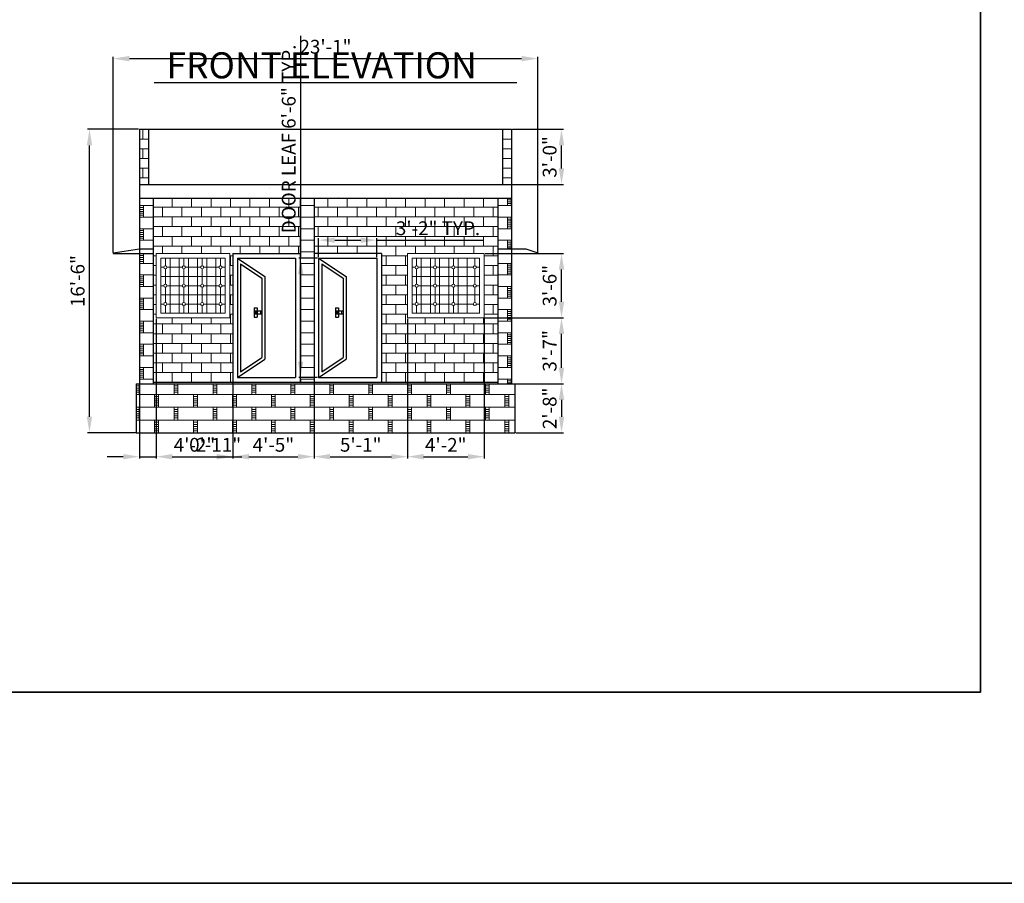
# Model space of a CAD drawing. Units: inches. Extents: x 1956 to 4770, y 1551 to 2596.
# Tile 8 of 10: x 2667 to 3310, y 1551 to 2115. Entities that reach past the tile are written whole.
import ezdxf

# ---------------------------------------------------------------- set-up
doc = ezdxf.new("R2010")
doc.units = ezdxf.units.IN
for name, color, linetype, lineweight in [('A-ANNO-DIMS', 2, 'Continuous', 18), ('A-ANNO-TITL', 6, 'Continuous', 25), ('A-ANNO-TTLB', 7, 'Continuous', 35), ('A-DOOR', 3, 'Continuous', 25), ('A-ELEV', 7, 'Continuous', 25), ('A-ELEV-PATT', 8, 'Continuous', 13), ('A-GLAZ', 4, 'Continuous', 18)]:
    doc.layers.add(name, color=color, linetype=linetype, lineweight=lineweight)
doc.styles.get("Standard").update_dxf_attribs({"font": 'arial.ttf'})
doc.dimstyles.new('ISO-25', dxfattribs={"dimtxt": 9, "dimasz": 10.5, "dimexe": 1.25, "dimexo": 0.625, "dimgap": 2, "dimtad": 1, "dimdec": 1, "dimlunit": 4, "dimtxsty": 'Standard', "dimcen": 2.5, "dimadec": 0, "dimazin": 0, "dimtfac": 1, "dimtdec": 1, "dimtmove": 0, "dimatfit": 3, "dimfxl": 1, "dimarcsym": 0})

# ---------------------------------------------------------------- blocks, each defined once
blk = doc.blocks.new('DOOR-ENTRY-PANEL-ELEV')
for p, q in [((0, 78), (38, 78)), ((0, 78), (0, 0)), ((0, 78), (18, 66)), ((38, 78), (38, 0)), ((2, 74.26), (16, 64.93)), ((2, 74.26), (2, 3.74)), ((16, 64.93), (16, 13.07)), ((18, 66), (18, 12)), ((11, 45.53), (11, 39.53)), ((11, 45.53), (13, 45.53)), ((13, 45.53), (13, 39.53)), ((11, 43.53), (16, 43.53)), ((11, 41.53), (16, 41.53)), ((11, 39.53), (13, 39.53)), ((12, 42.53), (11.64, 42.53)), ((12, 42.53), (12, 42.9)), ((12, 42.53), (12, 42.17)), ((12, 42.53), (12.36, 42.53)), ((15, 43.53), (15, 41.53)), ((16, 43.53), (16, 41.53)), ((2, 3.74), (16, 13.07)), ((0, 0), (18, 12)), ((0, 0), (38, 0))]:
    blk.add_line(p, q)
blk.add_circle((12, 42.53), 0.361)
blk = doc.blocks.new('*D41')
at = {"layer": 'A-ANNO-DIMS', "color": 0, "lineweight": -2, "transparency": 16777216}
for p, q in [((2850.27, 1959.25), (2850.27, 2104.31)), ((2861.35, 1959.25), (2849.02, 1959.25)), ((2850.27, 1891.75), (2850.27, 1948.75)), ((2861.35, 1881.25), (2849.02, 1881.25))]:
    blk.add_line(p, q, dxfattribs=at)
at = {"layer": 'A-ANNO-DIMS', "color": 0, "transparency": 16777216}
for points in [[(2848.52, 1948.75), (2852.02, 1948.75), (2850.27, 1959.25)], [(2848.52, 1891.75), (2852.02, 1891.75), (2850.27, 1881.25)]]:
    blk.add_solid(points, dxfattribs=at)
at = {"layer": 'Defpoints', "color": 0, "transparency": 16777216}
for p in [(2850.27, 1959.25), (2861.97, 1959.25), (2861.97, 1881.25)]:
    blk.add_point(p, dxfattribs=at)
at = {"layer": 'A-ANNO-DIMS', "color": 0, "transparency": 16777216, "insert": (2843.62, 2037.03), "char_height": 9, "attachment_point": 5, "rotation": 90}
blk.add_mtext('DOOR LEAF 6\'-6" TYP.', dxfattribs=at)
blk = doc.blocks.new('*D42')
at = {"layer": 'A-ANNO-DIMS', "color": 0, "lineweight": -2, "transparency": 16777216}
for p, q in [((2861.97, 1959.87), (2861.97, 1972.2)), ((2872.47, 1970.95), (2889.47, 1970.95)), ((2899.97, 1959.87), (2899.97, 1972.2)), ((2899.97, 1970.95), (2969.33, 1970.95))]:
    blk.add_line(p, q, dxfattribs=at)
at = {"layer": 'A-ANNO-DIMS', "color": 0, "transparency": 16777216}
for points in [[(2872.47, 1972.7), (2872.47, 1969.2), (2861.97, 1970.95)], [(2889.47, 1972.7), (2889.47, 1969.2), (2899.97, 1970.95)]]:
    blk.add_solid(points, dxfattribs=at)
at = {"layer": 'Defpoints', "color": 0, "transparency": 16777216}
for p in [(2899.97, 1970.95), (2861.97, 1959.25), (2899.97, 1959.25)]:
    blk.add_point(p, dxfattribs=at)
at = {"layer": 'A-ANNO-DIMS', "color": 0, "transparency": 16777216, "insert": (2939.9, 1977.55), "char_height": 9, "attachment_point": 5}
blk.add_mtext('3\'-2" TYP.', dxfattribs=at)
blk = doc.blocks.new('*D69')
at = {"layer": 'A-ANNO-DIMS', "color": 0, "lineweight": -2, "transparency": 16777216}
for p, q in [((2727.97, 1962.87), (2727.97, 2090.61)), ((2738.47, 2089.36), (2994.47, 2089.36)), ((3004.97, 1962.87), (3004.97, 2090.61))]:
    blk.add_line(p, q, dxfattribs=at)
at = {"layer": 'A-ANNO-DIMS', "color": 0, "transparency": 16777216}
for points in [[(2738.47, 2091.11), (2738.47, 2087.61), (2727.97, 2089.36)], [(2994.47, 2091.11), (2994.47, 2087.61), (3004.97, 2089.36)]]:
    blk.add_solid(points, dxfattribs=at)
at = {"layer": 'Defpoints', "color": 0, "transparency": 16777216}
for p in [(3004.97, 2089.36), (2727.97, 1962.25), (3004.97, 1962.25)]:
    blk.add_point(p, dxfattribs=at)
at = {"layer": 'A-ANNO-DIMS', "color": 0, "transparency": 16777216, "insert": (2866.47, 2095.95), "char_height": 9, "attachment_point": 5}
blk.add_mtext('23\'-1"', dxfattribs=at)
blk = doc.blocks.new('*D70')
at = {"layer": 'A-ANNO-DIMS', "color": 0, "lineweight": -2, "transparency": 16777216}
for p, q in [((2744.35, 2043.25), (2711.17, 2043.25)), ((2712.42, 1855.75), (2712.42, 2032.75)), ((2742.35, 1845.25), (2711.17, 1845.25))]:
    blk.add_line(p, q, dxfattribs=at)
at = {"layer": 'A-ANNO-DIMS', "color": 0, "transparency": 16777216}
for points in [[(2710.67, 2032.75), (2714.17, 2032.75), (2712.42, 2043.25)], [(2710.67, 1855.75), (2714.17, 1855.75), (2712.42, 1845.25)]]:
    blk.add_solid(points, dxfattribs=at)
at = {"layer": 'Defpoints', "color": 0, "transparency": 16777216}
for p in [(2712.42, 2043.25), (2744.97, 2043.25), (2742.97, 1845.25)]:
    blk.add_point(p, dxfattribs=at)
at = {"layer": 'A-ANNO-DIMS', "color": 0, "transparency": 16777216, "insert": (2705.83, 1944.25), "char_height": 9, "attachment_point": 5, "rotation": 90}
blk.add_mtext('16\'-6"', dxfattribs=at)
blk = doc.blocks.new('*D71')
at = {"layer": 'A-ANNO-DIMS', "color": 0, "lineweight": -2, "transparency": 16777216}
for p, q in [((2990.6, 1877.25), (3021.77, 1877.25)), ((3020.52, 1866.75), (3020.52, 1855.75)), ((2990.6, 1845.25), (3021.77, 1845.25))]:
    blk.add_line(p, q, dxfattribs=at)
at = {"layer": 'A-ANNO-DIMS', "color": 0, "transparency": 16777216}
for points in [[(3018.77, 1866.75), (3022.27, 1866.75), (3020.52, 1877.25)], [(3018.77, 1855.75), (3022.27, 1855.75), (3020.52, 1845.25)]]:
    blk.add_solid(points, dxfattribs=at)
at = {"layer": 'Defpoints', "color": 0, "transparency": 16777216}
for p in [(2989.97, 1877.25), (2989.97, 1845.25), (3020.52, 1845.25)]:
    blk.add_point(p, dxfattribs=at)
at = {"layer": 'A-ANNO-DIMS', "color": 0, "transparency": 16777216, "insert": (3013.93, 1861.25), "char_height": 9, "attachment_point": 5, "rotation": 90}
blk.add_mtext('2\'-8"', dxfattribs=at)
blk = doc.blocks.new('*D72')
at = {"layer": 'A-ANNO-DIMS', "color": 0, "lineweight": -2, "transparency": 16777216}
for p, q in [((2988.6, 2043.25), (3021.77, 2043.25)), ((3020.52, 2017.75), (3020.52, 2032.75)), ((2988.6, 2007.25), (3021.77, 2007.25))]:
    blk.add_line(p, q, dxfattribs=at)
at = {"layer": 'A-ANNO-DIMS', "color": 0, "transparency": 16777216}
for points in [[(3018.77, 2032.75), (3022.27, 2032.75), (3020.52, 2043.25)], [(3018.77, 2017.75), (3022.27, 2017.75), (3020.52, 2007.25)]]:
    blk.add_solid(points, dxfattribs=at)
at = {"layer": 'Defpoints', "color": 0, "transparency": 16777216}
for p in [(2987.97, 2043.25), (3020.52, 2043.25), (2987.97, 2007.25)]:
    blk.add_point(p, dxfattribs=at)
at = {"layer": 'A-ANNO-DIMS', "color": 0, "transparency": 16777216, "insert": (3013.93, 2025.25), "char_height": 9, "attachment_point": 5, "rotation": 90}
blk.add_mtext('3\'-0"', dxfattribs=at)
blk = doc.blocks.new('*D73')
at = {"layer": 'A-ANNO-DIMS', "color": 0, "lineweight": -2, "transparency": 16777216}
for p, q in [((2970.6, 1962.25), (3021.77, 1962.25)), ((3020.52, 1930.75), (3020.52, 1951.75)), ((2970.6, 1920.25), (3021.77, 1920.25))]:
    blk.add_line(p, q, dxfattribs=at)
at = {"layer": 'A-ANNO-DIMS', "color": 0, "transparency": 16777216}
for points in [[(3018.77, 1951.75), (3022.27, 1951.75), (3020.52, 1962.25)], [(3018.77, 1930.75), (3022.27, 1930.75), (3020.52, 1920.25)]]:
    blk.add_solid(points, dxfattribs=at)
at = {"layer": 'Defpoints', "color": 0, "transparency": 16777216}
for p in [(2969.97, 1962.25), (3020.52, 1962.25), (2969.97, 1920.25)]:
    blk.add_point(p, dxfattribs=at)
at = {"layer": 'A-ANNO-DIMS', "color": 0, "transparency": 16777216, "insert": (3013.93, 1941.25), "char_height": 9, "attachment_point": 5, "rotation": 90}
blk.add_mtext('3\'-6"', dxfattribs=at)
blk = doc.blocks.new('*D74')
at = {"layer": 'A-ANNO-DIMS', "color": 0, "lineweight": -2, "transparency": 16777216}
for p, q in [((2970.6, 1920.25), (3021.77, 1920.25)), ((3020.52, 1887.75), (3020.52, 1909.75)), ((2988.6, 1877.25), (3021.77, 1877.25))]:
    blk.add_line(p, q, dxfattribs=at)
at = {"layer": 'A-ANNO-DIMS', "color": 0, "transparency": 16777216}
for points in [[(3018.77, 1909.75), (3022.27, 1909.75), (3020.52, 1920.25)], [(3018.77, 1887.75), (3022.27, 1887.75), (3020.52, 1877.25)]]:
    blk.add_solid(points, dxfattribs=at)
at = {"layer": 'Defpoints', "color": 0, "transparency": 16777216}
for p in [(2969.97, 1920.25), (3020.52, 1920.25), (2987.97, 1877.25)]:
    blk.add_point(p, dxfattribs=at)
at = {"layer": 'A-ANNO-DIMS', "color": 0, "transparency": 16777216, "insert": (3013.93, 1898.75), "char_height": 9, "attachment_point": 5, "rotation": 90}
blk.add_mtext('3\'-7"', dxfattribs=at)
blk = doc.blocks.new('*D75')
at = {"layer": 'A-ANNO-DIMS', "color": 0, "lineweight": -2, "transparency": 16777216}
for p, q in [((2755.97, 1919.62), (2755.97, 1828.45)), ((2744.97, 1876.62), (2744.97, 1828.45)), ((2734.47, 1829.7), (2723.97, 1829.7)), ((2744.97, 1829.7), (2755.97, 1829.7)), ((2766.47, 1829.7), (2811.89, 1829.7))]:
    blk.add_line(p, q, dxfattribs=at)
at = {"layer": 'A-ANNO-DIMS', "color": 0, "transparency": 16777216}
for points in [[(2734.47, 1831.45), (2734.47, 1827.95), (2744.97, 1829.7)], [(2766.47, 1831.45), (2766.47, 1827.95), (2755.97, 1829.7)]]:
    blk.add_solid(points, dxfattribs=at)
at = {"layer": 'Defpoints', "color": 0, "transparency": 16777216}
for p in [(2755.97, 1920.25), (2744.97, 1877.25), (2755.97, 1829.7)]:
    blk.add_point(p, dxfattribs=at)
at = {"layer": 'A-ANNO-DIMS', "color": 0, "transparency": 16777216, "insert": (2794.43, 1836.29), "char_height": 9, "attachment_point": 5}
blk.add_mtext('0\'-11"', dxfattribs=at)
blk = doc.blocks.new('*D76')
at = {"layer": 'A-ANNO-DIMS', "color": 0, "lineweight": -2, "transparency": 16777216}
for p, q in [((2755.97, 1919.62), (2755.97, 1828.45)), ((2805.97, 1877.62), (2805.97, 1828.45)), ((2766.47, 1829.7), (2795.47, 1829.7))]:
    blk.add_line(p, q, dxfattribs=at)
at = {"layer": 'A-ANNO-DIMS', "color": 0, "transparency": 16777216}
for points in [[(2766.47, 1831.45), (2766.47, 1827.95), (2755.97, 1829.7)], [(2795.47, 1831.45), (2795.47, 1827.95), (2805.97, 1829.7)]]:
    blk.add_solid(points, dxfattribs=at)
at = {"layer": 'Defpoints', "color": 0, "transparency": 16777216}
for p in [(2755.97, 1920.25), (2805.97, 1878.25), (2805.97, 1829.7)]:
    blk.add_point(p, dxfattribs=at)
at = {"layer": 'A-ANNO-DIMS', "color": 0, "transparency": 16777216, "insert": (2780.97, 1836.22), "char_height": 9, "attachment_point": 5}
blk.add_mtext('4\'-2"', dxfattribs=at)
blk = doc.blocks.new('*D77')
at = {"layer": 'A-ANNO-DIMS', "color": 0, "lineweight": -2, "transparency": 16777216}
for p, q in [((2805.97, 1877.62), (2805.97, 1828.45)), ((2858.97, 1877.62), (2858.97, 1828.45)), ((2816.47, 1829.7), (2848.47, 1829.7))]:
    blk.add_line(p, q, dxfattribs=at)
at = {"layer": 'A-ANNO-DIMS', "color": 0, "transparency": 16777216}
for points in [[(2816.47, 1831.45), (2816.47, 1827.95), (2805.97, 1829.7)], [(2848.47, 1831.45), (2848.47, 1827.95), (2858.97, 1829.7)]]:
    blk.add_solid(points, dxfattribs=at)
at = {"layer": 'Defpoints', "color": 0, "transparency": 16777216}
for p in [(2805.97, 1878.25), (2858.97, 1878.25), (2858.97, 1829.7)]:
    blk.add_point(p, dxfattribs=at)
at = {"layer": 'A-ANNO-DIMS', "color": 0, "transparency": 16777216, "insert": (2832.47, 1836.28), "char_height": 9, "attachment_point": 5}
blk.add_mtext('4\'-5"', dxfattribs=at)
blk = doc.blocks.new('*D78')
at = {"layer": 'A-ANNO-DIMS', "color": 0, "lineweight": -2, "transparency": 16777216}
for p, q in [((2919.97, 1919.62), (2919.97, 1828.45)), ((2858.97, 1877.62), (2858.97, 1828.45)), ((2869.47, 1829.7), (2909.47, 1829.7))]:
    blk.add_line(p, q, dxfattribs=at)
at = {"layer": 'A-ANNO-DIMS', "color": 0, "transparency": 16777216}
for points in [[(2869.47, 1831.45), (2869.47, 1827.95), (2858.97, 1829.7)], [(2909.47, 1831.45), (2909.47, 1827.95), (2919.97, 1829.7)]]:
    blk.add_solid(points, dxfattribs=at)
at = {"layer": 'Defpoints', "color": 0, "transparency": 16777216}
for p in [(2919.97, 1920.25), (2858.97, 1878.25), (2919.97, 1829.7)]:
    blk.add_point(p, dxfattribs=at)
at = {"layer": 'A-ANNO-DIMS', "color": 0, "transparency": 16777216, "insert": (2889.47, 1836.29), "char_height": 9, "attachment_point": 5}
blk.add_mtext('5\'-1"', dxfattribs=at)
blk = doc.blocks.new('*D79')
at = {"layer": 'A-ANNO-DIMS', "color": 0, "lineweight": -2, "transparency": 16777216}
for p, q in [((2919.97, 1919.62), (2919.97, 1828.45)), ((2969.97, 1919.62), (2969.97, 1828.45)), ((2930.47, 1829.7), (2959.47, 1829.7))]:
    blk.add_line(p, q, dxfattribs=at)
at = {"layer": 'A-ANNO-DIMS', "color": 0, "transparency": 16777216}
for points in [[(2930.47, 1831.45), (2930.47, 1827.95), (2919.97, 1829.7)], [(2959.47, 1831.45), (2959.47, 1827.95), (2969.97, 1829.7)]]:
    blk.add_solid(points, dxfattribs=at)
at = {"layer": 'Defpoints', "color": 0, "transparency": 16777216}
for p in [(2919.97, 1920.25), (2969.97, 1920.25), (2969.97, 1829.7)]:
    blk.add_point(p, dxfattribs=at)
at = {"layer": 'A-ANNO-DIMS', "color": 0, "transparency": 16777216, "insert": (2944.97, 1836.22), "char_height": 9, "attachment_point": 5}
blk.add_mtext('4\'-2"', dxfattribs=at)

msp = doc.modelspace()

# ---------------------------------------------------------------- hatches: boundary and pattern name
at = {"layer": 'A-ELEV-PATT'}
h = msp.add_hatch(dxfattribs=at)
h.set_pattern_fill('BRICK', color=256)
h.set_pattern_definition([(0, (486.7216, 462.123), (0, 6.35), []), (90, (486.722, 462.123), (-12.7, 8e-16), [6.35, -6.35]), (90, (493.072, 462.123), (-12.7, 8e-16), [-6.35, 6.35])])
h.paths.add_polyline_path([(2805.97, 1962.25), (2849.97, 1962.25), (2849.97, 1998.25), (2753.97, 1998.25), (2753.97, 1878.25), (2805.97, 1878.25)])
h.paths.add_polyline_path([(2803.97, 1962.25), (2803.97, 1920.25), (2755.97, 1920.25), (2755.97, 1962.25)], flags=16)
h.paths.add_polyline_path([(2800.97, 1959.25), (2800.97, 1923.25), (2758.97, 1923.25), (2758.97, 1959.25)], flags=0)
h.paths.add_polyline_path([(2799, 1953.25, -0.414214), (2797.97, 1952.23), (2797.97, 1942.27, -0.414214), (2799, 1941.25, -0.414214), (2797.97, 1940.23), (2797.97, 1930.27, -0.414214), (2799, 1929.25, -1), (2796.95, 1929.25), (2787, 1929.25, -1), (2784.95, 1929.25), (2775, 1929.25, -1), (2772.95, 1929.25), (2763, 1929.25, -1), (2760.95, 1929.25, -0.414214), (2761.97, 1930.27), (2761.97, 1940.23, -0.414214), (2760.95, 1941.25, -0.414214), (2761.97, 1942.27), (2761.97, 1952.23, -0.414214), (2760.95, 1953.25, -1), (2763, 1953.25), (2772.95, 1953.25, -1), (2775, 1953.25), (2784.95, 1953.25, -1), (2787, 1953.25), (2796.95, 1953.25, -1)], flags=0)
h.paths.add_polyline_path([(2794.97, 1935.25), (2764.97, 1935.25), (2764.97, 1947.25), (2794.97, 1947.25)], flags=0)
h.paths.add_polyline_path([(2787, 1941.25, -1), (2784.95, 1941.25), (2775, 1941.25, -1), (2772.95, 1941.25, -1), (2775, 1941.25), (2784.95, 1941.25, -1)], flags=0)
h.paths.add_polyline_path([(2902.97, 1962.25), (2902.97, 1878.25), (2978.97, 1878.25), (2978.97, 1998.25), (2858.97, 1998.25), (2858.97, 1962.25)])
h.paths.add_polyline_path([(2919.97, 1962.25), (2969.97, 1962.25), (2969.97, 1920.25), (2919.97, 1920.25)], flags=16)
h.paths.add_polyline_path([(2922.97, 1959.25), (2966.97, 1959.25), (2966.97, 1923.25), (2922.97, 1923.25)], flags=0)
h.paths.add_polyline_path([(2927, 1953.25), (2936.95, 1953.25, -1), (2939, 1953.25), (2948.95, 1953.25, -1), (2951, 1953.25), (2962.95, 1953.25, -1), (2965, 1953.25, -0.414214), (2963.97, 1952.23), (2963.97, 1942.27, -0.414214), (2965, 1941.25, -0.414214), (2963.97, 1940.23), (2963.97, 1930.27, -0.414214), (2965, 1929.25, -1), (2962.95, 1929.25), (2951, 1929.25, -1), (2948.95, 1929.25), (2939, 1929.25, -1), (2936.95, 1929.25), (2927, 1929.25, -1), (2924.95, 1929.25, -0.414214), (2925.97, 1930.27), (2925.97, 1940.23, -0.414214), (2924.95, 1941.25, -0.414214), (2925.97, 1942.27), (2925.97, 1952.23, -0.414214), (2924.95, 1953.25, -1)], flags=0)
h.paths.add_polyline_path([(2928.97, 1947.25), (2958.97, 1947.25), (2958.97, 1935.25), (2928.97, 1935.25)], flags=0)
h.paths.add_polyline_path([(2939, 1941.25), (2948.95, 1941.25, -1), (2951, 1941.25, -1), (2948.95, 1941.25), (2939, 1941.25, -1), (2936.95, 1941.25, -1)], flags=0)
h.paths.add_polyline_path([(2750.97, 2043.25), (2744.97, 2043.25), (2744.97, 2007.25), (2750.97, 2007.25)])
h.paths.add_polyline_path([(2987.97, 2043.25), (2981.97, 2043.25), (2981.97, 2007.25), (2987.97, 2007.25)])
h = msp.add_hatch(dxfattribs=at)
h.set_pattern_fill('AR-CONC', color=256, scale=0.9)
h.set_pattern_definition([(50, (486.72, 462.12), (163.966, -14.345), [17.145, -188.595]), (355, (486.72, 462.12), (-31.719, 171.951), [13.716, -150.8765]), (100.4514, (500.39, 460.93), (132.247, 157.606), [14.571, -160.281]), (46.184, (486.72, 507.84), (243.971, -37.838), [25.718, -282.892]), (96.636, (507.05, 504.7), (213.664, 222.684), [21.857, -240.422]), (351.184, (486.72, 507.84), (213.664, 222.684), [20.574, -226.314]), (21, (509.58, 496.41), (136.453, -92.0387), [17.145, -188.595]), (326, (509.58, 496.41), (55.622, 165.769), [13.716, -150.876]), (71.4514, (520.95, 488.74), (192.075, 73.7305), [14.571, -160.281]), (37.5, (486.72, 462.123), (2.7797, 76.0995), [0, -149.0472, 0, -153.162, 0, -151.4475]), (7.5, (486.72, 462.12), (60.1377, 90.1625), [0, -87.3252, 0, -145.6182, 0, -57.7215]), (327.5, (435.744, 462.123), (122.0315, -5.1559), [0, -57.15, 0, -178.308, 0, -236.601]), (317.5, (412.88, 462.12), (133.3163, 22.884), [0, -74.295, 0, -118.4148, 0, -168.021])])
h.paths.add_polyline_path([(2849.97, 1998.25), (2987.97, 1998.25), (2987.97, 2007.25), (2744.97, 2007.25), (2744.97, 1998.25)])
h = msp.add_hatch(dxfattribs=at)
h.set_pattern_fill('BRSTONE', color=256, scale=0.9)
h.set_pattern_definition([(0, (486.7216, 462.123), (0, 7.5438), []), (90, (507.296, 462.123), (-11.43, 7.5438), [7.5438, -7.5438]), (90, (505.01, 462.123), (-11.43, 7.5438), [7.5438, -7.5438]), (0, (507.2956, 463.3805), (11.43, 7.5438), [-20.574, 2.286]), (0, (507.2956, 464.638), (11.43, 7.5438), [-20.574, 2.286]), (0, (507.2956, 465.895), (11.43, 7.5438), [-20.574, 2.286]), (0, (507.2956, 467.1524), (11.43, 7.5438), [-20.574, 2.286]), (0, (507.2956, 468.41), (11.43, 7.5438), [-20.574, 2.286])])
h.paths.add_polyline_path([(2744.97, 1877.25), (2753.97, 1877.25), (2753.97, 1962.25), (2744.97, 1962.25)])
h.paths.add_polyline_path([(2744.97, 1965.25), (2753.97, 1965.25), (2753.97, 1998.25), (2744.97, 1998.25)])
h.paths.add_polyline_path([(2849.97, 1998.25), (2849.97, 1878.25), (2858.97, 1878.25), (2858.97, 1998.25)])
h.paths.add_polyline_path([(2987.97, 1998.25), (2978.97, 1998.25), (2978.97, 1965.25), (2987.97, 1965.25)])
h.paths.add_polyline_path([(2978.97, 1877.25), (2987.97, 1877.25), (2987.97, 1962.25), (2978.97, 1962.25)])
h = msp.add_hatch(dxfattribs=at)
h.set_pattern_fill('BRSTONE', color=256)
h.set_pattern_definition([(0, (486.7216, 462.123), (0, 8.382), []), (90, (509.582, 462.123), (-12.7, 8.382), [8.382, -8.382]), (90, (507.042, 462.123), (-12.7, 8.382), [8.382, -8.382]), (0, (509.5816, 463.52), (12.7, 8.382), [-22.86, 2.54]), (0, (509.5816, 464.917), (12.7, 8.382), [-22.86, 2.54]), (0, (509.5816, 466.314), (12.7, 8.382), [-22.86, 2.54]), (0, (509.5816, 467.711), (12.7, 8.382), [-22.86, 2.54]), (0, (509.5816, 469.108), (12.7, 8.382), [-22.86, 2.54])])
h.paths.add_polyline_path([(2989.97, 1877.25), (2742.97, 1877.25), (2742.97, 1845.25), (2989.97, 1845.25)])

# ---------------------------------------------------------------- linework, layer by layer
at = {"layer": 'A-ANNO-TITL'}
msp.add_line((2754.74, 2073.81), (2991.37, 2073.81), dxfattribs=at)
at = {"layer": 'A-ANNO-TTLB'}
for points in [[(1955.79, 2596.29), (4769.89, 2596.29), (4769.89, 1551.4), (1955.79, 1551.4)], [(2042.64, 2439.33), (3293.93, 2439.33), (3293.93, 1676.04), (2042.64, 1676.04)]]:
    msp.add_lwpolyline(points, close=True, dxfattribs=at)
at = {"layer": 'A-DOOR'}
for p, q in [((2805.97, 1962.25), (2805.97, 1878.25)), ((2805.97, 1962.25), (2849.97, 1962.25)), ((2805.97, 1962.25), (2805.97, 1878.25)), ((2902.97, 1962.25), (2858.97, 1962.25)), ((2902.97, 1962.25), (2902.97, 1878.25))]:
    msp.add_line(p, q, dxfattribs=at)
at = {"layer": 'A-ELEV'}
for p, q in [((2744.97, 2043.25), (2744.97, 1877.25)), ((2744.97, 2043.25), (2987.97, 2043.25)), ((2750.97, 2043.25), (2750.97, 2007.25)), ((2981.97, 2043.25), (2981.97, 2007.25)), ((2987.97, 2043.25), (2987.97, 1877.25)), ((2744.97, 2007.25), (2987.97, 2007.25)), ((2744.97, 1998.25), (2849.97, 1998.25)), ((2753.97, 1998.25), (2753.97, 1877.25)), ((2849.97, 1998.25), (2849.97, 1878.25)), ((2849.97, 1998.25), (2987.97, 1998.25)), ((2858.97, 1998.25), (2858.97, 1878.25)), ((2978.97, 1998.25), (2978.97, 1877.25)), ((2727.97, 1962.75), (2744.97, 1965.25)), ((2727.97, 1962.75), (2727.97, 1962.25)), ((2727.97, 1962.25), (2753.97, 1962.25)), ((2744.97, 1965.25), (2753.97, 1965.25)), ((2978.97, 1965.25), (2997.25, 1965.25)), ((2978.97, 1962.25), (3004.97, 1962.25)), ((2997.25, 1965.25), (3004.97, 1962.75)), ((3004.97, 1962.75), (3004.97, 1962.25)), ((2969.97, 1920.25), (2987.97, 1920.25)), ((2742.97, 1877.25), (2989.97, 1877.25)), ((2742.97, 1877.25), (2742.97, 1845.25)), ((2753.97, 1878.25), (2978.97, 1878.25)), ((2987.97, 1877.25), (2989.97, 1877.25)), ((2989.97, 1877.25), (2989.97, 1845.25)), ((2742.97, 1845.25), (2989.97, 1845.25))]:
    msp.add_line(p, q, dxfattribs=at)
at = {"layer": 'A-GLAZ'}
for p, q in [((2755.97, 1962.25), (2803.97, 1962.25)), ((2755.97, 1962.25), (2755.97, 1920.25)), ((2803.97, 1962.25), (2803.97, 1920.25)), ((2919.97, 1962.25), (2969.97, 1962.25)), ((2919.97, 1962.25), (2919.97, 1920.25)), ((2969.97, 1962.25), (2969.97, 1920.25)), ((2758.97, 1959.25), (2800.97, 1959.25)), ((2758.97, 1959.25), (2758.97, 1923.25)), ((2761.97, 1959.25), (2761.97, 1954.27)), ((2764.97, 1959.25), (2764.97, 1923.25)), ((2770.97, 1959.25), (2770.97, 1923.25)), ((2773.97, 1959.25), (2773.97, 1954.27)), ((2776.97, 1959.25), (2776.97, 1923.25)), ((2782.97, 1959.25), (2782.97, 1923.25)), ((2785.97, 1959.25), (2785.97, 1954.27)), ((2788.97, 1959.25), (2788.97, 1923.25)), ((2794.97, 1959.25), (2794.97, 1923.25)), ((2797.97, 1959.25), (2797.97, 1954.27)), ((2800.97, 1959.25), (2800.97, 1923.25)), ((2922.97, 1959.25), (2966.97, 1959.25)), ((2922.97, 1959.25), (2922.97, 1923.25)), ((2925.97, 1959.25), (2925.97, 1954.27)), ((2928.97, 1959.25), (2928.97, 1923.25)), ((2934.97, 1959.25), (2934.97, 1923.25)), ((2937.97, 1959.25), (2937.97, 1954.27)), ((2940.97, 1959.25), (2940.97, 1923.25)), ((2946.97, 1959.25), (2946.97, 1923.25)), ((2949.97, 1959.25), (2949.97, 1954.27)), ((2952.97, 1959.25), (2952.97, 1923.25)), ((2958.97, 1959.25), (2958.97, 1923.25)), ((2963.97, 1959.25), (2963.97, 1954.27)), ((2966.97, 1959.25), (2966.97, 1923.25)), ((2758.97, 1953.25), (2760.95, 1953.25)), ((2761.97, 1952.23), (2761.97, 1942.27)), ((2763, 1953.25), (2772.95, 1953.25)), ((2773.97, 1952.23), (2773.97, 1942.27)), ((2775, 1953.25), (2784.95, 1953.25)), ((2785.97, 1952.23), (2785.97, 1942.27)), ((2787, 1953.25), (2796.95, 1953.25)), ((2797.97, 1952.23), (2797.97, 1942.27)), ((2799, 1953.25), (2800.97, 1953.25)), ((2922.97, 1953.25), (2924.95, 1953.25)), ((2925.97, 1952.23), (2925.97, 1942.27)), ((2927, 1953.25), (2936.95, 1953.25)), ((2937.97, 1952.23), (2937.97, 1942.27)), ((2939, 1953.25), (2948.95, 1953.25)), ((2949.97, 1952.23), (2949.97, 1942.27)), ((2951, 1953.25), (2962.95, 1953.25)), ((2963.97, 1952.23), (2963.97, 1942.27)), ((2965, 1953.25), (2966.97, 1953.25)), ((2758.97, 1947.25), (2800.97, 1947.25)), ((2758.97, 1941.25), (2760.95, 1941.25)), ((2763, 1941.25), (2772.95, 1941.25)), ((2775, 1941.25), (2784.95, 1941.25)), ((2787, 1941.25), (2796.95, 1941.25)), ((2799, 1941.25), (2800.97, 1941.25)), ((2922.97, 1947.25), (2966.97, 1947.25)), ((2922.97, 1941.25), (2924.95, 1941.25)), ((2927, 1941.25), (2936.95, 1941.25)), ((2939, 1941.25), (2948.95, 1941.25)), ((2951, 1941.25), (2962.95, 1941.25)), ((2965, 1941.25), (2966.97, 1941.25)), ((2758.97, 1935.25), (2800.97, 1935.25)), ((2761.97, 1940.23), (2761.97, 1930.27)), ((2773.97, 1940.23), (2773.97, 1930.27)), ((2785.97, 1940.23), (2785.97, 1930.27)), ((2797.97, 1940.23), (2797.97, 1930.27)), ((2922.97, 1935.25), (2966.97, 1935.25)), ((2925.97, 1940.23), (2925.97, 1930.27)), ((2937.97, 1940.23), (2937.97, 1930.27)), ((2949.97, 1940.23), (2949.97, 1930.27)), ((2963.97, 1940.23), (2963.97, 1930.27)), ((2758.97, 1929.25), (2760.95, 1929.25)), ((2761.97, 1928.23), (2761.97, 1923.25)), ((2763, 1929.25), (2772.95, 1929.25)), ((2773.97, 1928.23), (2773.97, 1923.25)), ((2775, 1929.25), (2784.95, 1929.25)), ((2785.97, 1928.23), (2785.97, 1923.25)), ((2787, 1929.25), (2796.95, 1929.25)), ((2797.97, 1928.23), (2797.97, 1923.25)), ((2799, 1929.25), (2800.97, 1929.25)), ((2922.97, 1929.25), (2924.95, 1929.25)), ((2925.97, 1928.23), (2925.97, 1923.25)), ((2927, 1929.25), (2936.95, 1929.25)), ((2937.97, 1928.23), (2937.97, 1923.25)), ((2939, 1929.25), (2948.95, 1929.25)), ((2949.97, 1928.23), (2949.97, 1923.25)), ((2951, 1929.25), (2962.95, 1929.25)), ((2965, 1929.25), (2966.97, 1929.25)), ((2758.97, 1923.25), (2800.97, 1923.25)), ((2922.97, 1923.25), (2966.97, 1923.25)), ((2755.97, 1920.25), (2803.97, 1920.25)), ((2919.97, 1920.25), (2969.97, 1920.25))]:
    msp.add_line(p, q, dxfattribs=at)
for centre in [(2761.97, 1953.25), (2773.97, 1953.25), (2785.97, 1953.25), (2797.97, 1953.25), (2925.97, 1953.25), (2937.97, 1953.25), (2949.97, 1953.25), (2963.97, 1953.25), (2761.97, 1941.25), (2773.97, 1941.25), (2785.97, 1941.25), (2797.97, 1941.25), (2925.97, 1941.25), (2937.97, 1941.25), (2949.97, 1941.25), (2963.97, 1941.25), (2761.97, 1929.25), (2773.97, 1929.25), (2785.97, 1929.25), (2797.97, 1929.25), (2925.97, 1929.25), (2937.97, 1929.25), (2949.97, 1929.25), (2963.97, 1929.25)]:
    msp.add_circle(centre, 1.02, dxfattribs=at)

# ---------------------------------------------------------------- block references
at = {"layer": 'A-DOOR'}
for p in [(2808.97, 1881.25), (2861.97, 1881.25)]:
    msp.add_blockref('DOOR-ENTRY-PANEL-ELEV', p, dxfattribs=at)

# ---------------------------------------------------------------- texts
at = {"layer": 'A-ANNO-TITL'}
msp.add_text(' FRONT ELEVATION ', height=17, dxfattribs=at).set_placement((2757.42, 2076.5))

# ---------------------------------------------------------------- dimensions: what is measured, and where the dimension line sits
at = {"layer": 'A-ANNO-DIMS'}
for base, p1, p2, picture, middle in [((3004.97, 2089.36), (2727.97, 1962.25), (3004.97, 1962.25), '*D69', (2866.47, 2095.95)), ((2755.97, 1829.7), (2744.97, 1877.25), (2755.97, 1920.25), '*D75', (2794.43, 1836.29)), ((2805.97, 1829.7), (2755.97, 1920.25), (2805.97, 1878.25), '*D76', (2780.97, 1836.22)), ((2919.97, 1829.7), (2858.97, 1878.25), (2919.97, 1920.25), '*D78', (2889.47, 1836.29)), ((2969.97, 1829.7), (2919.97, 1920.25), (2969.97, 1920.25), '*D79', (2944.97, 1836.22)), ((2858.97, 1829.7), (2805.97, 1878.25), (2858.97, 1878.25), '*D77', (2832.47, 1836.28))]:
    dim = msp.add_linear_dim(base=base, p1=p1, p2=p2, dimstyle='ISO-25', override={"dimdec": 1, "dimlfac": 1, "dimrnd": 0, "dimzin": 1, "dimdsep": 46, "dimlunit": 4, "dimfrac": 2}, dxfattribs=at)
    dim.commit()
    dim.dimension.update_dxf_attribs({"geometry": picture, "text_midpoint": middle})
dim = msp.add_linear_dim(base=(2850.27, 1959.25), p1=(2861.97, 1881.25), p2=(2861.97, 1959.25), angle=90, text='DOOR LEAF <> TYP.', dimstyle='ISO-25', override={"dimdec": 1, "dimlfac": 1, "dimrnd": 0, "dimzin": 1, "dimdsep": 46, "dimlunit": 4, "dimfrac": 2}, dxfattribs=at)
dim.commit()
dim.dimension.update_dxf_attribs({"geometry": '*D41', "text_midpoint": (2843.62, 2037.03)})
for base, p1, p2, picture, middle in [((2712.42, 2043.25), (2742.97, 1845.25), (2744.97, 2043.25), '*D70', (2705.83, 1944.25)), ((3020.52, 2043.25), (2987.97, 2007.25), (2987.97, 2043.25), '*D72', (3013.93, 2025.25)), ((3020.52, 1962.25), (2969.97, 1920.25), (2969.97, 1962.25), '*D73', (3013.93, 1941.25)), ((3020.52, 1920.25), (2987.97, 1877.25), (2969.97, 1920.25), '*D74', (3013.93, 1898.75)), ((3020.52, 1845.25), (2989.97, 1877.25), (2989.97, 1845.25), '*D71', (3013.93, 1861.25))]:
    dim = msp.add_linear_dim(base=base, p1=p1, p2=p2, angle=90, dimstyle='ISO-25', override={"dimdec": 1, "dimlfac": 1, "dimrnd": 0, "dimzin": 1, "dimdsep": 46, "dimlunit": 4, "dimfrac": 2}, dxfattribs=at)
    dim.commit()
    dim.dimension.update_dxf_attribs({"geometry": picture, "text_midpoint": middle})
dim = msp.add_linear_dim(base=(2899.97, 1970.95), p1=(2861.97, 1959.25), p2=(2899.97, 1959.25), text='<> TYP.', dimstyle='ISO-25', override={"dimdec": 1, "dimlfac": 1, "dimrnd": 0, "dimzin": 1, "dimdsep": 46, "dimlunit": 4, "dimfrac": 2}, dxfattribs=at)
dim.commit()
dim.dimension.update_dxf_attribs({"geometry": '*D42', "text_midpoint": (2939.9, 1977.55)})

doc.saveas('drawing.dxf')
